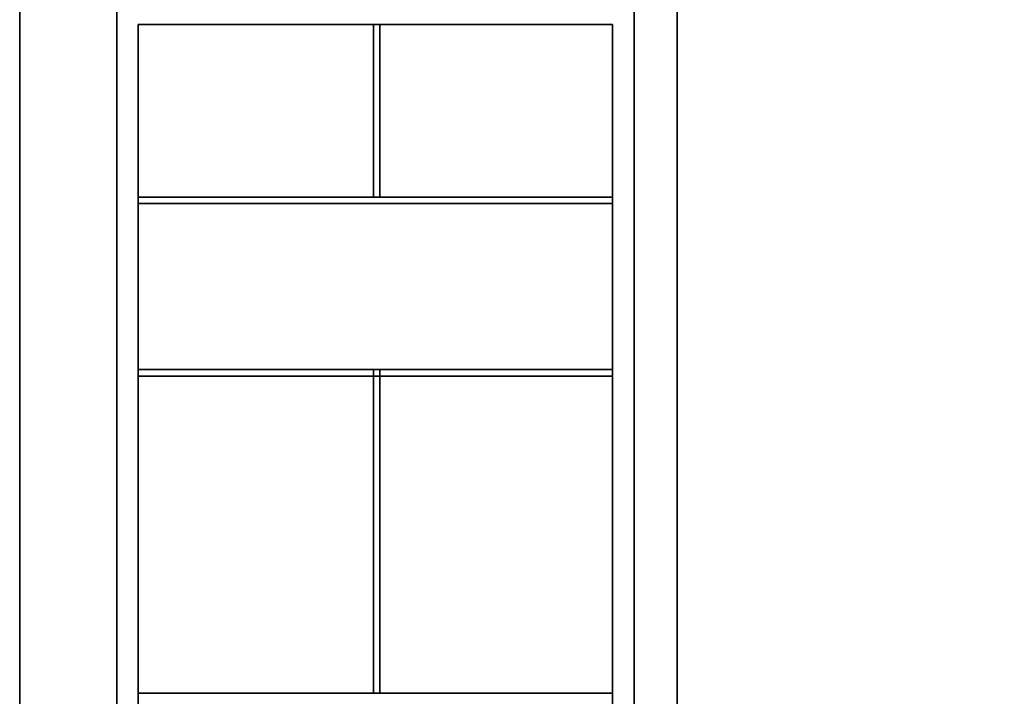
# Model space of a CAD drawing. Units: inches. Extents: x 64 to 1167, y 117 to 939.
# Tile 35 of 56: x 983 to 1074, y 476 to 539. Entities that reach past the tile are written whole.
import ezdxf

# ---------------------------------------------------------------- set-up
doc = ezdxf.new("R2010")
doc.units = ezdxf.units.IN
doc.header["$MEASUREMENT"] = 0
doc.layers.add('A-SECT', color=7, linetype='Continuous', lineweight=35)

msp = doc.modelspace()

# ---------------------------------------------------------------- linework, layer by layer
at = {"layer": 'A-SECT'}
for p, q in [((991.813, 556.679), (991.813, 436.679)), ((1039.813, 540.679), (1039.813, 436.679)), ((1043.813, 540.679), (1043.813, 436.679)), ((993.813, 538.679), (993.813, 436.679)), ((1037.813, 538.679), (993.813, 538.679)), ((1015.631, 538.679), (1015.631, 522.679)), ((1016.231, 538.679), (1016.231, 522.679)), ((1037.813, 538.679), (1037.813, 436.679)), ((1037.813, 522.679), (993.813, 522.679)), ((1037.813, 522.079), (993.813, 522.079)), ((1037.813, 506.679), (993.813, 506.679)), ((1037.813, 506.079), (993.813, 506.079)), ((1015.631, 506.679), (1015.631, 476.679)), ((1016.231, 506.679), (1016.231, 476.679)), ((1037.813, 476.679), (993.813, 476.679))]:
    msp.add_line(p, q, dxfattribs=at)
msp.add_lwpolyline([(982.813, 427.679), (1166.813, 427.679), (1166.813, 565.679), (982.813, 565.679)], close=True, dxfattribs=at)

doc.saveas('drawing.dxf')
